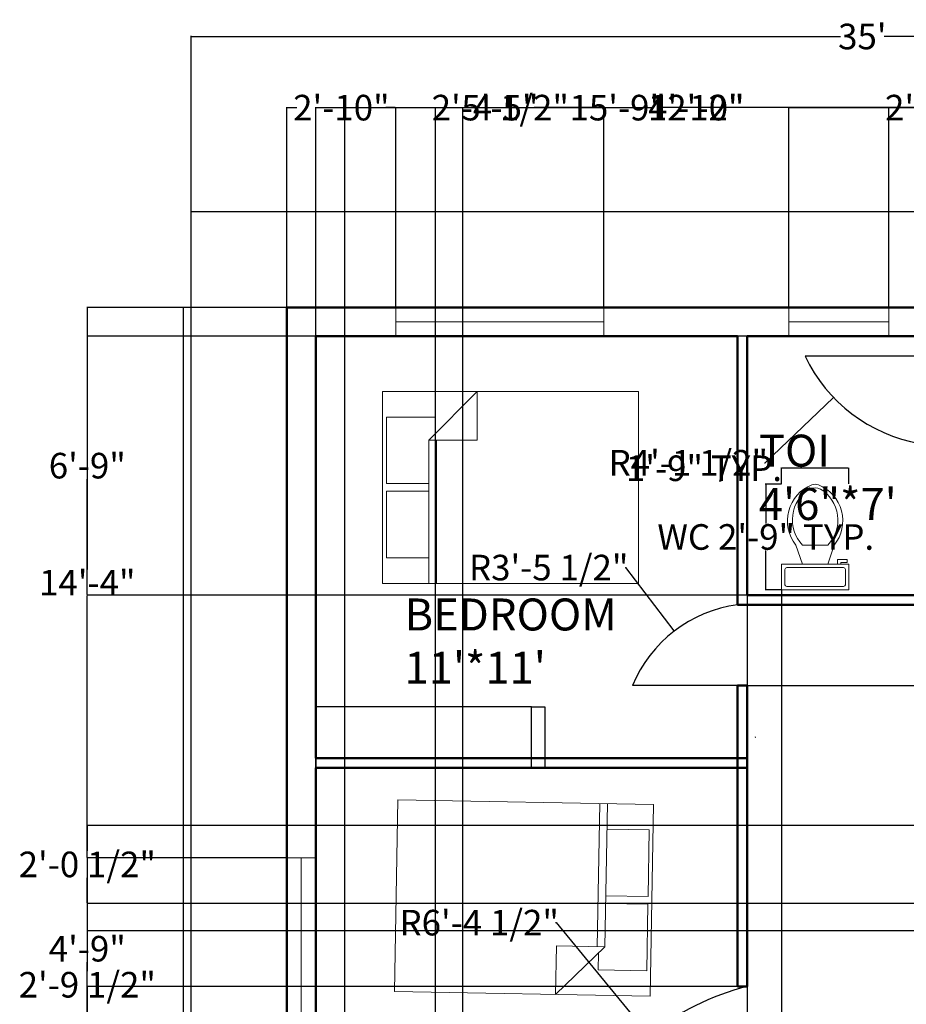
# Model space of a CAD drawing. Units: inches. Extents: x 3437 to 3994, y 3379 to 4084.
# Tile 5 of 6: x 3437 to 3715, y 3776 to 4084. Entities that reach past the tile are written whole.
import ezdxf

# ---------------------------------------------------------------- set-up
doc = ezdxf.new("R2010")
doc.units = ezdxf.units.IN
doc.header["$MEASUREMENT"] = 0
for name, color, linetype, lineweight in [('A-ANNO-DIMS', 2, 'Continuous', 18), ('A-AREA-IDEN', 7, 'Continuous', 25), ('A-DOOR', 3, 'Continuous', 25), ('A-FLOR-CASE', 8, 'Continuous', 25), ('A-FLOR-FIXT', 9, 'Continuous', 18), ('A-FURN', 8, 'Continuous', 18), ('A-GLAZ', 4, 'Continuous', 18), ('A-WALL', 7, 'Continuous', 50), ('C-PROP', 3, 'Continuous', 25)]:
    doc.layers.add(name, color=color, linetype=linetype, lineweight=lineweight)
doc.styles.get("Standard").update_dxf_attribs({"font": 'arial.ttf'})
doc.dimstyles.get("Standard").update_dxf_attribs({"dimtxt": 8, "dimasz": 0.18, "dimexe": 0.18, "dimexo": 0.0625, "dimgap": 0.09, "dimtad": 0, "dimtih": 1, "dimtoh": 1, "dimdec": 0, "dimzin": 0, "dimdsep": 46, "dimlunit": 3, "dimtxsty": 'Standard', "dimcen": 0.09, "dimadec": 0, "dimazin": 0, "dimtfac": 1, "dimtdec": 0, "dimtofl": 0, "dimtmove": 0, "dimatfit": 3, "dimfxl": 1, "dimtolj": 1, "dimtzin": 0, "dimarcsym": 0})

# ---------------------------------------------------------------- blocks, each defined once
blk = doc.blocks.new('Bed - Queen')
for p, q in [((0, -80.00003), (0, 0)), ((0, 0), (59.99999, 0)), ((59.99999, 0), (59.99999, -80.00003)), ((7.99999, -1.2), (28.79998, -1.2)), ((7.99999, -14.4), (7.99999, -1.2)), ((28.79998, -1.2), (28.79998, -14.4)), ((31.19999, -1.2), (51.99999, -1.2)), ((31.19999, -14.4), (31.19999, -1.2)), ((51.99999, -1.2), (51.99999, -16.4)), ((0, -14.4), (44.8, -14.4)), ((59.99999, -29.6), (44.8, -14.4)), ((44.8, -14.4), (44.8, -29.6)), ((44.8, -16.8), (0, -16.8)), ((51.99999, -16.4), (46.79936, -16.4)), ((44.8, -29.6), (59.99999, -29.6)), ((59.99999, -80.00003), (0, -80.00003))]:
    blk.add_line(p, q)
blk = doc.blocks.new('Toilet - top')
for p, q in [((9.5, -6), (9.5, -2)), ((-10, -8.5), (-8, -8.5)), ((-10, -9.5), (-10, -8.5)), ((-8, -8.5), (-8, -8)), ((-7, -8), (-7, -9.5)), ((-4, -8), (-6, -14)), ((4, -8), (6, -14)), ((-7, -9.5), (-10, -9.5)), ((4, -14), (-4, -14))]:
    blk.add_line(p, q)
blk.add_lwpolyline([(10.5, -8), (10.5, 0), (-10.5, 0), (-10.5, -8)], close=True)
for points in [[(-9.5, -2), (-9.5, -6)], [(8.5, -1), (-8.5, -1)], [(-8.5, -7), (8.5, -7)]]:
    blk.add_lwpolyline(points)
for centre, radius, start, end in [((-8.62, -1.88), 0.884, 81.8699, 188.1301), ((8.62, -1.88), 0.884, 351.8699, 98.1301), ((-8.62, -6.12), 0.884, 171.8699, 278.1301), ((8.62, -6.12), 0.884, 261.8699, 8.1301), ((3.52, -21.58), 12.17, 141.4691, 247.9714), ((4.2, -21.82), 11.33, 136.3677, 238.9468), ((-3.52, -21.58), 12.17, 292.0284, 38.5307), ((-4.2, -21.82), 11.33, 301.053, 43.6321), ((0, -27.88), 4, 245.7318, 294.2682), ((0, -29), 4, 254.8605, 285.1395)]:
    blk.add_arc(centre, radius, start, end)
blk = doc.blocks.new('*D9')
at = {"layer": 'A-ANNO-DIMS', "color": 0, "lineweight": -2, "transparency": 16777216}
for p, q in [((3491.02, 4023.7), (3491.02, 4078.52)), ((3491.2, 4078.34), (3694.15, 4078.34)), ((3910.84, 4078.34), (3707.9, 4078.34)), ((3911.02, 4023.7), (3911.02, 4078.52))]:
    blk.add_line(p, q, dxfattribs=at)
at = {"layer": 'A-ANNO-DIMS', "color": 0, "transparency": 16777216}
for points in [[(3491.2, 4078.37), (3491.2, 4078.31), (3491.02, 4078.34)], [(3910.84, 4078.37), (3910.84, 4078.31), (3911.02, 4078.34)]]:
    blk.add_solid(points, dxfattribs=at)
at = {"layer": 'Defpoints', "color": 0, "transparency": 16777216}
for p in [(3911.02, 4078.34), (3491.02, 4023.64), (3911.02, 4023.64)]:
    blk.add_point(p, dxfattribs=at)
at = {"layer": 'A-ANNO-DIMS', "color": 0, "transparency": 16777216, "insert": (3701.02, 4078.34), "char_height": 8, "attachment_point": 5}
blk.add_mtext("\\A1;35'", dxfattribs=at)
blk = doc.blocks.new('*D15')
at = {"layer": 'A-ANNO-DIMS', "color": 0, "lineweight": -2, "transparency": 16777216}
for p, q in [((3675.7, 3938.36), (3670.62, 3938.36)), ((3670.8, 3938.18), (3670.8, 3926.06)), ((3670.8, 3905.49), (3670.8, 3917.61)), ((3675.7, 3905.31), (3670.62, 3905.31))]:
    blk.add_line(p, q, dxfattribs=at)
at = {"layer": 'A-ANNO-DIMS', "color": 0, "transparency": 16777216}
for points in [[(3670.77, 3938.18), (3670.83, 3938.18), (3670.8, 3938.36)], [(3670.77, 3905.49), (3670.83, 3905.49), (3670.8, 3905.31)]]:
    blk.add_solid(points, dxfattribs=at)
at = {"layer": 'Defpoints', "color": 0, "transparency": 16777216}
for p in [(3675.76, 3938.36), (3670.8, 3905.31), (3675.76, 3905.31)]:
    blk.add_point(p, dxfattribs=at)
at = {"layer": 'A-ANNO-DIMS', "color": 0, "transparency": 16777216, "insert": (3670.8, 3921.84), "char_height": 8, "attachment_point": 5}
blk.add_mtext('\\A1;WC 2\'-9" TYP.', dxfattribs=at)
blk = doc.blocks.new('*D16')
at = {"layer": 'A-ANNO-DIMS', "color": 0, "lineweight": -2, "transparency": 16777216}
for p, q in [((3675.76, 3943.32), (3675.58, 3943.32)), ((3675.76, 3938.42), (3675.76, 3943.5)), ((3696.58, 3943.32), (3675.94, 3943.32)), ((3696.76, 3938.42), (3696.76, 3943.5))]:
    blk.add_line(p, q, dxfattribs=at)
at = {"layer": 'A-ANNO-DIMS', "color": 0, "transparency": 16777216}
for points in [[(3675.94, 3943.35), (3675.94, 3943.29), (3675.76, 3943.32)], [(3696.58, 3943.35), (3696.58, 3943.29), (3696.76, 3943.32)]]:
    blk.add_solid(points, dxfattribs=at)
at = {"layer": 'Defpoints', "color": 0, "transparency": 16777216}
for p in [(3675.76, 3943.32), (3675.76, 3938.36), (3696.76, 3938.36)]:
    blk.add_point(p, dxfattribs=at)
at = {"layer": 'A-ANNO-DIMS', "color": 0, "transparency": 16777216, "insert": (3651.48, 3943.32), "char_height": 8, "attachment_point": 5}
blk.add_mtext('\\A1;1\'-9" TYP.', dxfattribs=at)
blk = doc.blocks.new('*D28')
at = {"layer": 'A-ANNO-DIMS', "color": 0, "lineweight": -2, "transparency": 16777216}
for p, q in [((3520.96, 3993.64), (3488.39, 3993.64)), ((3488.57, 3993.46), (3488.57, 3712.81)), ((3488.57, 3423.82), (3488.57, 3704.46)), ((3520.96, 3423.64), (3488.39, 3423.64))]:
    blk.add_line(p, q, dxfattribs=at)
at = {"layer": 'A-ANNO-DIMS', "color": 0, "transparency": 16777216}
for points in [[(3488.54, 3993.46), (3488.6, 3993.46), (3488.57, 3993.64)], [(3488.54, 3423.82), (3488.6, 3423.82), (3488.57, 3423.64)]]:
    blk.add_solid(points, dxfattribs=at)
at = {"layer": 'Defpoints', "color": 0, "transparency": 16777216}
for p in [(3488.57, 3993.64), (3521.02, 3993.64), (3521.02, 3423.64)]:
    blk.add_point(p, dxfattribs=at)
at = {"layer": 'A-ANNO-DIMS', "color": 0, "transparency": 16777216, "insert": (3488.57, 3708.64), "char_height": 8, "attachment_point": 5}
blk.add_mtext('\\A1;47\'-6"', dxfattribs=at)
blk = doc.blocks.new('*D29')
at = {"layer": 'A-ANNO-DIMS', "color": 0, "lineweight": -2, "transparency": 16777216}
for p, q in [((3521.02, 3993.7), (3521.02, 4056.27)), ((3521.2, 4056.09), (3524.16, 4056.09)), ((3554.92, 4056.09), (3551.96, 4056.09)), ((3555.1, 3993.7), (3555.1, 4056.27))]:
    blk.add_line(p, q, dxfattribs=at)
at = {"layer": 'A-ANNO-DIMS', "color": 0, "transparency": 16777216}
for points in [[(3521.2, 4056.12), (3521.2, 4056.06), (3521.02, 4056.09)], [(3554.92, 4056.12), (3554.92, 4056.06), (3555.1, 4056.09)]]:
    blk.add_solid(points, dxfattribs=at)
at = {"layer": 'Defpoints', "color": 0, "transparency": 16777216}
for p in [(3555.1, 4056.09), (3521.02, 3993.64), (3555.1, 3993.64)]:
    blk.add_point(p, dxfattribs=at)
at = {"layer": 'A-ANNO-DIMS', "color": 0, "transparency": 16777216, "insert": (3538.06, 4056.09), "char_height": 8, "attachment_point": 5}
blk.add_mtext('\\A1;2\'-10"', dxfattribs=at)
blk = doc.blocks.new('*D30')
at = {"layer": 'A-ANNO-DIMS', "color": 0, "lineweight": -2, "transparency": 16777216}
for p, q in [((3555.1, 3993.7), (3555.1, 4056.27)), ((3555.28, 4056.09), (3576.93, 4056.09)), ((3620.01, 4056.09), (3598.37, 4056.09)), ((3620.19, 3993.7), (3620.19, 4056.27))]:
    blk.add_line(p, q, dxfattribs=at)
at = {"layer": 'A-ANNO-DIMS', "color": 0, "transparency": 16777216}
for points in [[(3555.28, 4056.12), (3555.28, 4056.06), (3555.1, 4056.09)], [(3620.01, 4056.12), (3620.01, 4056.06), (3620.19, 4056.09)]]:
    blk.add_solid(points, dxfattribs=at)
at = {"layer": 'Defpoints', "color": 0, "transparency": 16777216}
for p in [(3620.19, 4056.09), (3555.1, 3993.64), (3620.19, 3993.64)]:
    blk.add_point(p, dxfattribs=at)
at = {"layer": 'A-ANNO-DIMS', "color": 0, "transparency": 16777216, "insert": (3587.65, 4056.09), "char_height": 8, "attachment_point": 5}
blk.add_mtext('\\A1;5\'-5"', dxfattribs=at)
blk = doc.blocks.new('*D31')
at = {"layer": 'A-ANNO-DIMS', "color": 0, "lineweight": -2, "transparency": 16777216}
for p, q in [((3620.19, 3993.7), (3620.19, 4056.27)), ((3620.37, 4056.09), (3635.11, 4056.09)), ((3677.84, 4056.09), (3663.1, 4056.09)), ((3678.02, 3993.7), (3678.02, 4056.27))]:
    blk.add_line(p, q, dxfattribs=at)
at = {"layer": 'A-ANNO-DIMS', "color": 0, "transparency": 16777216}
for points in [[(3620.37, 4056.12), (3620.37, 4056.06), (3620.19, 4056.09)], [(3677.84, 4056.12), (3677.84, 4056.06), (3678.02, 4056.09)]]:
    blk.add_solid(points, dxfattribs=at)
at = {"layer": 'Defpoints', "color": 0, "transparency": 16777216}
for p in [(3678.02, 4056.09), (3620.19, 3993.64), (3678.02, 3993.64)]:
    blk.add_point(p, dxfattribs=at)
at = {"layer": 'A-ANNO-DIMS', "color": 0, "transparency": 16777216, "insert": (3649.11, 4056.09), "char_height": 8, "attachment_point": 5}
blk.add_mtext('\\A1;4\'-10"', dxfattribs=at)
blk = doc.blocks.new('*D32')
at = {"layer": 'A-ANNO-DIMS', "color": 0, "lineweight": -2, "transparency": 16777216}
for p, q in [((3678.02, 3993.7), (3678.02, 4056.27)), ((3678.2, 4056.09), (3709.13, 4056.09)), ((3709.31, 3993.7), (3709.31, 4056.27)), ((3709.31, 4056.09), (3709.49, 4056.09))]:
    blk.add_line(p, q, dxfattribs=at)
at = {"layer": 'A-ANNO-DIMS', "color": 0, "transparency": 16777216}
for points in [[(3678.2, 4056.12), (3678.2, 4056.06), (3678.02, 4056.09)], [(3709.13, 4056.12), (3709.13, 4056.06), (3709.31, 4056.09)]]:
    blk.add_solid(points, dxfattribs=at)
at = {"layer": 'Defpoints', "color": 0, "transparency": 16777216}
for p in [(3709.31, 4056.09), (3678.02, 3993.64), (3709.31, 3993.64)]:
    blk.add_point(p, dxfattribs=at)
at = {"layer": 'A-ANNO-DIMS', "color": 0, "transparency": 16777216, "insert": (3729.6, 4056.09), "char_height": 8, "attachment_point": 5}
blk.add_mtext('\\A1;2\'-7 1/2"', dxfattribs=at)
blk = doc.blocks.new('*D33')
at = {"layer": 'A-ANNO-DIMS', "color": 0, "lineweight": -2, "transparency": 16777216}
for p, q in [((3709.31, 3993.7), (3709.31, 4056.27)), ((3709.49, 4056.09), (3729.7, 4056.09)), ((3771.35, 4056.09), (3751.14, 4056.09)), ((3771.53, 3993.7), (3771.53, 4056.27))]:
    blk.add_line(p, q, dxfattribs=at)
at = {"layer": 'A-ANNO-DIMS', "color": 0, "transparency": 16777216}
for points in [[(3709.49, 4056.12), (3709.49, 4056.06), (3709.31, 4056.09)], [(3771.35, 4056.12), (3771.35, 4056.06), (3771.53, 4056.09)]]:
    blk.add_solid(points, dxfattribs=at)
at = {"layer": 'Defpoints', "color": 0, "transparency": 16777216}
for p in [(3771.53, 4056.09), (3709.31, 3993.64), (3771.53, 3993.64)]:
    blk.add_point(p, dxfattribs=at)
at = {"layer": 'A-ANNO-DIMS', "color": 0, "transparency": 16777216, "insert": (3740.42, 4056.09), "char_height": 8, "attachment_point": 5}
blk.add_mtext('\\A1;5\'-2"', dxfattribs=at)
blk = doc.blocks.new('*D35')
at = {"layer": 'A-ANNO-DIMS', "color": 0, "lineweight": -2, "transparency": 16777216}
for p, q in [((3520.96, 3993.64), (3458.39, 3993.64)), ((3458.57, 3993.46), (3458.57, 3911.67)), ((3458.57, 3821.66), (3458.57, 3903.45)), ((3520.96, 3821.48), (3458.39, 3821.48))]:
    blk.add_line(p, q, dxfattribs=at)
at = {"layer": 'A-ANNO-DIMS', "color": 0, "transparency": 16777216}
for points in [[(3458.54, 3993.46), (3458.6, 3993.46), (3458.57, 3993.64)], [(3458.54, 3821.66), (3458.6, 3821.66), (3458.57, 3821.48)]]:
    blk.add_solid(points, dxfattribs=at)
at = {"layer": 'Defpoints', "color": 0, "transparency": 16777216}
for p in [(3521.02, 3993.64), (3458.57, 3821.48), (3521.02, 3821.48)]:
    blk.add_point(p, dxfattribs=at)
at = {"layer": 'A-ANNO-DIMS', "color": 0, "transparency": 16777216, "insert": (3458.57, 3907.56), "char_height": 8, "attachment_point": 5}
blk.add_mtext('\\A1;14\'-4"', dxfattribs=at)
blk = doc.blocks.new('*D36')
at = {"layer": 'A-ANNO-DIMS', "color": 0, "lineweight": -2, "transparency": 16777216}
for p, q in [((3520.96, 3821.48), (3458.39, 3821.48)), ((3458.57, 3821.3), (3458.57, 3797.26)), ((3458.57, 3764.87), (3458.57, 3788.91)), ((3520.96, 3764.69), (3458.39, 3764.69))]:
    blk.add_line(p, q, dxfattribs=at)
at = {"layer": 'A-ANNO-DIMS', "color": 0, "transparency": 16777216}
for points in [[(3458.54, 3821.3), (3458.6, 3821.3), (3458.57, 3821.48)], [(3458.54, 3764.87), (3458.6, 3764.87), (3458.57, 3764.69)]]:
    blk.add_solid(points, dxfattribs=at)
at = {"layer": 'Defpoints', "color": 0, "transparency": 16777216}
for p in [(3521.02, 3821.48), (3458.57, 3764.69), (3521.02, 3764.69)]:
    blk.add_point(p, dxfattribs=at)
at = {"layer": 'A-ANNO-DIMS', "color": 0, "transparency": 16777216, "insert": (3458.57, 3793.09), "char_height": 8, "attachment_point": 5}
blk.add_mtext('\\A1;4\'-9"', dxfattribs=at)
blk = doc.blocks.new('*D46')
at = {"layer": 'A-ANNO-DIMS', "color": 0, "lineweight": -2, "transparency": 16777216}
for p, q in [((3576.02, 3426.7), (3576.02, 4056.27)), ((3576.2, 4056.09), (3635.57, 4056.09)), ((3721.84, 4056.09), (3662.48, 4056.09)), ((3722.02, 3426.7), (3722.02, 4056.27))]:
    blk.add_line(p, q, dxfattribs=at)
at = {"layer": 'A-ANNO-DIMS', "color": 0, "transparency": 16777216}
for points in [[(3576.2, 4056.12), (3576.2, 4056.06), (3576.02, 4056.09)], [(3721.84, 4056.12), (3721.84, 4056.06), (3722.02, 4056.09)]]:
    blk.add_solid(points, dxfattribs=at)
at = {"layer": 'Defpoints', "color": 0, "transparency": 16777216}
for p in [(3722.02, 4056.09), (3576.02, 3426.64), (3722.02, 3426.64)]:
    blk.add_point(p, dxfattribs=at)
at = {"layer": 'A-ANNO-DIMS', "color": 0, "transparency": 16777216, "insert": (3649.02, 4056.09), "char_height": 8, "attachment_point": 5}
blk.add_mtext('\\A1;12\'-2"', dxfattribs=at)
blk = doc.blocks.new('*D47')
at = {"layer": 'A-ANNO-DIMS', "color": 0, "lineweight": -2, "transparency": 16777216}
for p, q in [((3521.02, 3993.57), (3521.02, 3391.01)), ((3530.02, 3984.57), (3530.02, 3391.01)), ((3521.2, 3391.19), (3529.84, 3391.19)), ((3530.02, 3391.19), (3530.2, 3391.19))]:
    blk.add_line(p, q, dxfattribs=at)
at = {"layer": 'A-ANNO-DIMS', "color": 0, "transparency": 16777216}
for points in [[(3521.2, 3391.22), (3521.2, 3391.16), (3521.02, 3391.19)], [(3529.84, 3391.22), (3529.84, 3391.16), (3530.02, 3391.19)]]:
    blk.add_solid(points, dxfattribs=at)
at = {"layer": 'Defpoints', "color": 0, "transparency": 16777216}
for p in [(3521.02, 3993.64), (3530.02, 3984.64), (3530.02, 3391.19)]:
    blk.add_point(p, dxfattribs=at)
at = {"layer": 'A-ANNO-DIMS', "color": 0, "transparency": 16777216, "insert": (3540.93, 3391.19), "char_height": 8, "attachment_point": 5}
blk.add_mtext('\\A1;0\'-9"', dxfattribs=at)
blk = doc.blocks.new('*D49')
at = {"layer": 'A-ANNO-DIMS', "color": 0, "lineweight": -2, "transparency": 16777216}
for p, q in [((3530.02, 3504.7), (3530.02, 4056.27)), ((3530.2, 4056.09), (3611.07, 4056.09)), ((3718.84, 4056.09), (3637.98, 4056.09)), ((3719.02, 3504.7), (3719.02, 4056.27))]:
    blk.add_line(p, q, dxfattribs=at)
at = {"layer": 'A-ANNO-DIMS', "color": 0, "transparency": 16777216}
for points in [[(3530.2, 4056.12), (3530.2, 4056.06), (3530.02, 4056.09)], [(3718.84, 4056.12), (3718.84, 4056.06), (3719.02, 4056.09)]]:
    blk.add_solid(points, dxfattribs=at)
at = {"layer": 'Defpoints', "color": 0, "transparency": 16777216}
for p in [(3719.02, 4056.09), (3530.02, 3504.64), (3719.02, 3504.64)]:
    blk.add_point(p, dxfattribs=at)
at = {"layer": 'A-ANNO-DIMS', "color": 0, "transparency": 16777216, "insert": (3624.52, 4056.09), "char_height": 8, "attachment_point": 5}
blk.add_mtext('\\A1;15\'-9"', dxfattribs=at)
blk = doc.blocks.new('*D55')
at = {"layer": 'A-ANNO-DIMS', "color": 0, "lineweight": -2, "transparency": 16777216}
for p, q in [((3662.09, 3900.64), (3943.65, 3900.64)), ((3943.47, 3900.46), (3943.47, 3892.12)), ((3943.47, 3875.57), (3943.47, 3883.91)), ((3662.09, 3875.39), (3943.65, 3875.39))]:
    blk.add_line(p, q, dxfattribs=at)
at = {"layer": 'A-ANNO-DIMS', "color": 0, "transparency": 16777216}
for points in [[(3943.44, 3900.46), (3943.5, 3900.46), (3943.47, 3900.64)], [(3943.44, 3875.57), (3943.5, 3875.57), (3943.47, 3875.39)]]:
    blk.add_solid(points, dxfattribs=at)
at = {"layer": 'Defpoints', "color": 0, "transparency": 16777216}
for p in [(3662.02, 3900.64), (3662.02, 3875.39), (3943.47, 3875.39)]:
    blk.add_point(p, dxfattribs=at)
at = {"layer": 'A-ANNO-DIMS', "color": 0, "transparency": 16777216, "insert": (3943.47, 3888.01), "char_height": 8, "attachment_point": 5}
blk.add_mtext('\\A1;2\'-1"', dxfattribs=at)
blk = doc.blocks.new('*D58')
at = {"layer": 'A-ANNO-DIMS', "color": 0, "lineweight": -2, "transparency": 16777216}
for p, q in [((3775.96, 3831.64), (3458.39, 3831.64)), ((3458.57, 3831.46), (3458.57, 3823.68)), ((3458.57, 3807.45), (3458.57, 3815.23)), ((3775.96, 3807.27), (3458.39, 3807.27))]:
    blk.add_line(p, q, dxfattribs=at)
at = {"layer": 'A-ANNO-DIMS', "color": 0, "transparency": 16777216}
for points in [[(3458.54, 3831.46), (3458.6, 3831.46), (3458.57, 3831.64)], [(3458.54, 3807.45), (3458.6, 3807.45), (3458.57, 3807.27)]]:
    blk.add_solid(points, dxfattribs=at)
at = {"layer": 'Defpoints', "color": 0, "transparency": 16777216}
for p in [(3776.02, 3831.64), (3458.57, 3807.27), (3776.02, 3807.27)]:
    blk.add_point(p, dxfattribs=at)
at = {"layer": 'A-ANNO-DIMS', "color": 0, "transparency": 16777216, "insert": (3458.57, 3819.45), "char_height": 8, "attachment_point": 5}
blk.add_mtext('\\A1;2\'-0 1/2"', dxfattribs=at)
blk = doc.blocks.new('*D59')
at = {"layer": 'A-ANNO-DIMS', "color": 0, "lineweight": -2, "transparency": 16777216}
for p, q in [((3661.96, 3781.25), (3458.39, 3781.25)), ((3458.57, 3781.07), (3458.57, 3764.22)), ((3458.57, 3738.92), (3458.57, 3755.76)), ((3661.96, 3738.74), (3458.39, 3738.74))]:
    blk.add_line(p, q, dxfattribs=at)
at = {"layer": 'A-ANNO-DIMS', "color": 0, "transparency": 16777216}
for points in [[(3458.54, 3781.07), (3458.6, 3781.07), (3458.57, 3781.25)], [(3458.54, 3738.92), (3458.6, 3738.92), (3458.57, 3738.74)]]:
    blk.add_solid(points, dxfattribs=at)
at = {"layer": 'Defpoints', "color": 0, "transparency": 16777216}
for p in [(3662.02, 3781.25), (3458.57, 3738.74), (3662.02, 3738.74)]:
    blk.add_point(p, dxfattribs=at)
at = {"layer": 'A-ANNO-DIMS', "color": 0, "transparency": 16777216, "insert": (3458.57, 3759.99), "char_height": 8, "attachment_point": 5}
blk.add_mtext('\\A1;3\'-6 1/2"', dxfattribs=at)
blk = doc.blocks.new('*D60')
at = {"layer": 'A-ANNO-DIMS', "color": 0, "lineweight": -2, "transparency": 16777216}
for p, q in [((3539.11, 3729.7), (3539.11, 4056.27)), ((3539.29, 4056.09), (3567.31, 4056.09)), ((3567.49, 3729.7), (3567.49, 4056.27)), ((3567.49, 4056.09), (3567.67, 4056.09))]:
    blk.add_line(p, q, dxfattribs=at)
at = {"layer": 'A-ANNO-DIMS', "color": 0, "transparency": 16777216}
for points in [[(3539.29, 4056.12), (3539.29, 4056.06), (3539.11, 4056.09)], [(3567.31, 4056.12), (3567.31, 4056.06), (3567.49, 4056.09)]]:
    blk.add_solid(points, dxfattribs=at)
at = {"layer": 'Defpoints', "color": 0, "transparency": 16777216}
for p in [(3567.49, 4056.09), (3539.11, 3729.64), (3567.49, 3729.64)]:
    blk.add_point(p, dxfattribs=at)
at = {"layer": 'A-ANNO-DIMS', "color": 0, "transparency": 16777216, "insert": (3587.78, 4056.09), "char_height": 8, "attachment_point": 5}
blk.add_mtext('\\A1;2\'-4 1/2"', dxfattribs=at)
blk = doc.blocks.new('*D79')
at = {"layer": 'A-ANNO-DIMS', "color": 0, "lineweight": -2, "transparency": 16777216}
for p, q in [((3675.76, 3905.25), (3675.76, 3391.01)), ((3665.02, 3903.57), (3665.02, 3391.01)), ((3665.2, 3391.19), (3675.58, 3391.19)), ((3675.76, 3391.19), (3675.94, 3391.19))]:
    blk.add_line(p, q, dxfattribs=at)
at = {"layer": 'A-ANNO-DIMS', "color": 0, "transparency": 16777216}
for points in [[(3665.2, 3391.22), (3665.2, 3391.16), (3665.02, 3391.19)], [(3675.58, 3391.22), (3675.58, 3391.16), (3675.76, 3391.19)]]:
    blk.add_solid(points, dxfattribs=at)
at = {"layer": 'Defpoints', "color": 0, "transparency": 16777216}
for p in [(3675.76, 3905.31), (3665.02, 3903.64), (3675.76, 3391.19)]:
    blk.add_point(p, dxfattribs=at)
at = {"layer": 'A-ANNO-DIMS', "color": 0, "transparency": 16777216, "insert": (3699.09, 3391.19), "char_height": 8, "attachment_point": 5}
blk.add_mtext('\\A1;0\'-10 1/2"', dxfattribs=at)
blk = doc.blocks.new('*D80')
at = {"layer": 'A-ANNO-DIMS', "color": 0, "lineweight": -2, "transparency": 16777216}
for p, q in [((3664.96, 3984.64), (3458.39, 3984.64)), ((3458.57, 3984.46), (3458.57, 3948.31)), ((3458.57, 3903.82), (3458.57, 3939.96)), ((3664.96, 3903.64), (3458.39, 3903.64))]:
    blk.add_line(p, q, dxfattribs=at)
at = {"layer": 'A-ANNO-DIMS', "color": 0, "transparency": 16777216}
for points in [[(3458.54, 3984.46), (3458.6, 3984.46), (3458.57, 3984.64)], [(3458.54, 3903.82), (3458.6, 3903.82), (3458.57, 3903.64)]]:
    blk.add_solid(points, dxfattribs=at)
at = {"layer": 'Defpoints', "color": 0, "transparency": 16777216}
for p in [(3665.02, 3984.64), (3458.57, 3903.64), (3665.02, 3903.64)]:
    blk.add_point(p, dxfattribs=at)
at = {"layer": 'A-ANNO-DIMS', "color": 0, "transparency": 16777216, "insert": (3458.57, 3944.14), "char_height": 8, "attachment_point": 5}
blk.add_mtext('\\A1;6\'-9"', dxfattribs=at)
blk = doc.blocks.new('*D86')
at = {"layer": 'A-ANNO-DIMS', "color": 0, "lineweight": -2, "transparency": 16777216}
for p, q in [((3775.96, 3798.64), (3458.39, 3798.64)), ((3458.57, 3798.46), (3458.57, 3786.05)), ((3458.57, 3765.19), (3458.57, 3777.6)), ((3791.17, 3765.01), (3458.39, 3765.01))]:
    blk.add_line(p, q, dxfattribs=at)
at = {"layer": 'A-ANNO-DIMS', "color": 0, "transparency": 16777216}
for points in [[(3458.54, 3798.46), (3458.6, 3798.46), (3458.57, 3798.64)], [(3458.54, 3765.19), (3458.6, 3765.19), (3458.57, 3765.01)]]:
    blk.add_solid(points, dxfattribs=at)
at = {"layer": 'Defpoints', "color": 0, "transparency": 16777216}
for p in [(3776.02, 3798.64), (3458.57, 3765.01), (3791.23, 3765.01)]:
    blk.add_point(p, dxfattribs=at)
at = {"layer": 'A-ANNO-DIMS', "color": 0, "transparency": 16777216, "insert": (3458.57, 3781.82), "char_height": 8, "attachment_point": 5}
blk.add_mtext('\\A1;2\'-9 1/2"', dxfattribs=at)
blk = doc.blocks.new('*D87')
at = {"layer": 'A-ANNO-DIMS', "color": 0, "lineweight": -2, "transparency": 16777216}
for p, q in [((3605.04, 3801.24), (3605.22, 3801.24)), ((3605.22, 3801.24), (3634.29, 3766.05)), ((3682.97, 3707.03), (3683.15, 3707.03)), ((3683.06, 3706.94), (3683.06, 3707.12))]:
    blk.add_line(p, q, dxfattribs=at)
at = {"layer": 'A-ANNO-DIMS', "color": 0, "transparency": 16777216}
blk.add_solid([(3634.32, 3766.07), (3634.27, 3766.03), (3634.41, 3765.91)], dxfattribs=at)
at = {"layer": 'Defpoints', "color": 0, "transparency": 16777216}
for p in [(3634.41, 3765.91), (3683.06, 3707.03)]:
    blk.add_point(p, dxfattribs=at)
at = {"layer": 'A-ANNO-DIMS', "color": 0, "transparency": 16777216, "insert": (3581.17, 3801.24), "char_height": 8, "attachment_point": 5}
blk.add_mtext('\\A1;R6\'-4 1/2"', dxfattribs=at)
blk = doc.blocks.new('*D91')
at = {"layer": 'A-ANNO-DIMS', "color": 0, "lineweight": -2, "transparency": 16777216}
for p, q in [((3626.79, 3912.27), (3626.97, 3912.27)), ((3626.97, 3912.27), (3642.08, 3892.54)), ((3667.47, 3859.29), (3667.65, 3859.29)), ((3667.56, 3859.2), (3667.56, 3859.38))]:
    blk.add_line(p, q, dxfattribs=at)
at = {"layer": 'A-ANNO-DIMS', "color": 0, "transparency": 16777216}
blk.add_solid([(3642.1, 3892.56), (3642.06, 3892.53), (3642.19, 3892.4)], dxfattribs=at)
at = {"layer": 'Defpoints', "color": 0, "transparency": 16777216}
for p in [(3642.19, 3892.4), (3667.56, 3859.29)]:
    blk.add_point(p, dxfattribs=at)
at = {"layer": 'A-ANNO-DIMS', "color": 0, "transparency": 16777216, "insert": (3602.91, 3912.27), "char_height": 8, "attachment_point": 5}
blk.add_mtext('\\A1;R3\'-5 1/2"', dxfattribs=at)
blk = doc.blocks.new('*D95')
at = {"layer": 'A-ANNO-DIMS', "color": 0, "lineweight": -2, "transparency": 16777216}
for p, q in [((3727.49, 3999.57), (3727.67, 3999.57)), ((3727.58, 3999.48), (3727.58, 3999.66)), ((3670.64, 3945.04), (3691.86, 3965.37)), ((3670.46, 3945.04), (3670.64, 3945.04))]:
    blk.add_line(p, q, dxfattribs=at)
at = {"layer": 'A-ANNO-DIMS', "color": 0, "transparency": 16777216}
blk.add_solid([(3691.84, 3965.39), (3691.88, 3965.34), (3691.99, 3965.49)], dxfattribs=at)
at = {"layer": 'Defpoints', "color": 0, "transparency": 16777216}
for p in [(3727.58, 3999.57), (3691.99, 3965.49)]:
    blk.add_point(p, dxfattribs=at)
at = {"layer": 'A-ANNO-DIMS', "color": 0, "transparency": 16777216, "insert": (3646.59, 3945.04), "char_height": 8, "attachment_point": 5}
blk.add_mtext('\\A1;R4\'-1 1/2"', dxfattribs=at)

msp = doc.modelspace()

# ---------------------------------------------------------------- linework, layer by layer
at = {"layer": 'A-DOOR'}
for p, q in [((3719.02, 3978.34), (3683.11, 3978.34)), ((3662.02, 3875.39), (3629.08, 3875.39))]:
    msp.add_line(p, q, dxfattribs=at)
for centre, radius, start, end in [((3727.58, 3999.57), 49.27, 205.5271, 260.0037), ((3667.56, 3859.29), 41.71, 97.6285, 157.2996), ((3683.06, 3707.03), 76.38, 103.6573, 155.4718)]:
    msp.add_arc(centre, radius, start, end, dxfattribs=at)
at = {"layer": 'A-FLOR-CASE'}
for p, q in [((3597.52, 3868.68), (3530.02, 3868.68)), ((3597.52, 3849.64), (3597.52, 3868.68)), ((3597.52, 3868.68), (3601.67, 3868.68)), ((3601.67, 3868.68), (3601.67, 3849.64))]:
    msp.add_line(p, q, dxfattribs=at)
at = {"layer": 'A-GLAZ'}
for p, q in [((3555.1, 3993.64), (3555.1, 3984.64)), ((3620.19, 3993.64), (3620.19, 3984.64)), ((3678.02, 3993.64), (3678.02, 3984.64)), ((3709.31, 3993.64), (3709.31, 3984.64)), ((3555.1, 3989.14), (3620.19, 3989.14)), ((3678.02, 3989.14), (3709.31, 3989.14)), ((3521.02, 3821.48), (3530.02, 3821.48)), ((3525.52, 3821.48), (3525.52, 3764.69))]:
    msp.add_line(p, q, dxfattribs=at)
at = {"layer": 'A-WALL'}
for p, q in [((3521.02, 3423.64), (3521.02, 3993.64)), ((3521.02, 3993.64), (3881.02, 3993.64)), ((3530.02, 3984.64), (3662.02, 3984.64)), ((3530.02, 3852.64), (3530.02, 3984.64)), ((3662.02, 3900.64), (3662.02, 3984.64)), ((3665.02, 3984.64), (3872.02, 3984.64)), ((3665.02, 3903.64), (3665.02, 3984.64)), ((3665.02, 3903.64), (3719.02, 3903.64)), ((3665.02, 3900.64), (3662.02, 3900.64)), ((3665.02, 3900.64), (3722.02, 3900.64)), ((3665.02, 3875.39), (3662.02, 3875.39)), ((3662.02, 3875.39), (3662.02, 3861.38)), ((3665.02, 3861.38), (3665.02, 3875.39)), ((3662.02, 3781.25), (3662.02, 3861.38)), ((3665.02, 3781.25), (3665.02, 3861.38)), ((3530.02, 3852.64), (3665.02, 3852.64)), ((3530.02, 3849.64), (3665.02, 3849.64)), ((3530.02, 3729.64), (3530.02, 3849.64)), ((3662.02, 3781.25), (3665.02, 3781.25))]:
    msp.add_line(p, q, dxfattribs=at)
at = {"layer": 'C-PROP'}
msp.add_lwpolyline([(3770.9, 3423.64), (3491.02, 3423.64), (3491.02, 4023.64), (3911.02, 4023.64), (3911.02, 3423.64), (3890.36, 3423.64)], dxfattribs=at)

# ---------------------------------------------------------------- block references
at = {"layer": 'A-FLOR-FIXT', "rotation": 180}
msp.add_blockref('Toilet - top', (3686.26, 3905.31), dxfattribs=at)
at = {"layer": 'A-FURN'}
for p, rotation in [((3550.96, 3907.32), 90), ((3635.73, 3838.19), 268.9520281987376)]:
    msp.add_blockref('Bed - Queen', p, dxfattribs=dict(at, rotation=rotation))

# ---------------------------------------------------------------- texts
at = {"layer": 'A-AREA-IDEN', "char_height": 10, "attachment_point": 1}
for s, insert in [('TOI\\P4\'6"*7\'', (3668.66, 3953.82)), ("BEDROOM\\P11'*11'", (3557.8, 3902.6))]:
    msp.add_mtext_dynamic_manual_height_columns(s, width=200.853, gutter_width=1, heights=[0], dxfattribs=dict(at, insert=insert))

# ---------------------------------------------------------------- dimensions: what is measured, and where the dimension line sits
at = {"layer": 'A-ANNO-DIMS'}
for base, p1, p2, override, picture, middle in [((3911.02, 4078.34), (3491.02, 4023.64), (3911.02, 4023.64), {"dimclrd": 0, "dimclre": 0, "dimclrt": 0}, '*D9', (3701.02, 4078.34)), ((3567.49, 4056.09), (3539.11, 3729.64), (3567.49, 3729.64), {"dimdec": 1, "dimlfac": 1, "dimrnd": 0, "dimzin": 1, "dimdsep": 46, "dimlunit": 4, "dimfrac": 2}, '*D60', (3587.78, 4056.09)), ((3709.31, 4056.09), (3678.02, 3993.64), (3709.31, 3993.64), {"dimdec": 1, "dimlfac": 1, "dimrnd": 0, "dimzin": 1, "dimdsep": 46, "dimlunit": 4, "dimfrac": 2}, '*D32', (3729.6, 4056.09)), ((3555.1, 4056.09), (3521.02, 3993.64), (3555.1, 3993.64), {"dimdec": 1, "dimlfac": 1, "dimrnd": 0, "dimzin": 1, "dimdsep": 46, "dimlunit": 4, "dimfrac": 2}, '*D29', (3538.06, 4056.09)), ((3719.02, 4056.09), (3530.02, 3504.64), (3719.02, 3504.64), {"dimdec": 1, "dimlfac": 1, "dimrnd": 0, "dimzin": 1, "dimdsep": 46, "dimlunit": 4, "dimfrac": 2}, '*D49', (3624.52, 4056.09)), ((3620.19, 4056.09), (3555.1, 3993.64), (3620.19, 3993.64), {"dimdec": 1, "dimlfac": 1, "dimrnd": 0, "dimzin": 1, "dimdsep": 46, "dimlunit": 4, "dimfrac": 2}, '*D30', (3587.65, 4056.09)), ((3722.02, 4056.09), (3576.02, 3426.64), (3722.02, 3426.64), {"dimdec": 1, "dimlfac": 1, "dimrnd": 0, "dimzin": 1, "dimdsep": 46, "dimlunit": 4, "dimfrac": 2}, '*D46', (3649.02, 4056.09)), ((3678.02, 4056.09), (3620.19, 3993.64), (3678.02, 3993.64), {"dimdec": 1, "dimlfac": 1, "dimrnd": 0, "dimzin": 1, "dimdsep": 46, "dimlunit": 4, "dimfrac": 2}, '*D31', (3649.11, 4056.09)), ((3771.53, 4056.09), (3709.31, 3993.64), (3771.53, 3993.64), {"dimdec": 1, "dimlfac": 1, "dimrnd": 0, "dimzin": 1, "dimdsep": 46, "dimlunit": 4, "dimfrac": 2}, '*D33', (3740.42, 4056.09)), ((3530.02, 3391.19), (3521.02, 3993.64), (3530.02, 3984.64), {"dimdec": 1, "dimlfac": 1, "dimrnd": 0, "dimzin": 1, "dimdsep": 46, "dimlunit": 4, "dimfrac": 2}, '*D47', (3540.93, 3391.19)), ((3675.76, 3391.19), (3665.02, 3903.64), (3675.76, 3905.31), {"dimdec": 1, "dimlfac": 1, "dimrnd": 0, "dimzin": 1, "dimdsep": 46, "dimlunit": 4, "dimfrac": 2}, '*D79', (3699.09, 3391.19))]:
    dim = msp.add_linear_dim(base=base, p1=p1, p2=p2, dimstyle='Standard', override=override, dxfattribs=at)
    dim.commit()
    dim.dimension.update_dxf_attribs({"geometry": picture, "text_midpoint": middle})
for center, mpoint, picture, middle in [((3727.58, 3999.57), (3691.99, 3965.49), '*D95', (3646.59, 3945.04)), ((3667.56, 3859.29), (3642.19, 3892.4), '*D91', (3602.91, 3912.27)), ((3683.06, 3707.03), (3634.41, 3765.91), '*D87', (3581.17, 3801.24))]:
    dim = msp.add_radius_dim(center=center, mpoint=mpoint, dimstyle='Standard', override={"dimdec": 1, "dimlfac": 1, "dimrnd": 0, "dimzin": 1, "dimdsep": 46, "dimlunit": 4, "dimfrac": 2}, dxfattribs=at)
    dim.commit()
    dim.dimension.update_dxf_attribs({"geometry": picture, "text_midpoint": middle, "dimtype": 164})
for base, p1, p2, picture, middle in [((3458.57, 3821.48), (3521.02, 3993.64), (3521.02, 3821.48), '*D35', (3458.57, 3907.56)), ((3488.57, 3993.64), (3521.02, 3423.64), (3521.02, 3993.64), '*D28', (3488.57, 3708.64)), ((3458.57, 3903.64), (3665.02, 3984.64), (3665.02, 3903.64), '*D80', (3458.57, 3944.14)), ((3943.4743, 3875.389), (3662.0243, 3900.6359), (3662.0243, 3875.389), '*D55', (3943.4743, 3888.0125)), ((3458.57, 3807.27), (3776.02, 3831.64), (3776.02, 3807.27), '*D58', (3458.57, 3819.45)), ((3458.57, 3764.69), (3521.02, 3821.48), (3521.02, 3764.69), '*D36', (3458.57, 3793.09)), ((3458.57, 3765.01), (3776.02, 3798.64), (3791.23, 3765.01), '*D86', (3458.57, 3781.82)), ((3458.57, 3738.74), (3662.02, 3781.25), (3662.02, 3738.74), '*D59', (3458.57, 3759.99))]:
    dim = msp.add_linear_dim(base=base, p1=p1, p2=p2, angle=90, dimstyle='Standard', override={"dimdec": 1, "dimlfac": 1, "dimrnd": 0, "dimzin": 1, "dimdsep": 46, "dimlunit": 4, "dimfrac": 2}, dxfattribs=at)
    dim.commit()
    dim.dimension.update_dxf_attribs({"geometry": picture, "text_midpoint": middle})
for base, p1, p2, angle, text, picture, middle in [((3675.76, 3943.32), (3696.76, 3938.36), (3675.76, 3938.36), 180, '<> TYP.', '*D16', (3651.48, 3943.32)), ((3670.8014, 3905.313), (3675.7584, 3938.3592), (3675.7584, 3905.313), 270, 'WC <> TYP.', '*D15', (3670.8014, 3921.8361))]:
    dim = msp.add_linear_dim(base=base, p1=p1, p2=p2, angle=angle, text=text, dimstyle='Standard', override={"dimdec": 1, "dimlfac": 1, "dimrnd": 0, "dimzin": 1, "dimdsep": 46, "dimlunit": 4, "dimfrac": 2}, dxfattribs=at)
    dim.commit()
    dim.dimension.update_dxf_attribs({"geometry": picture, "text_midpoint": middle})

doc.saveas('drawing.dxf')
